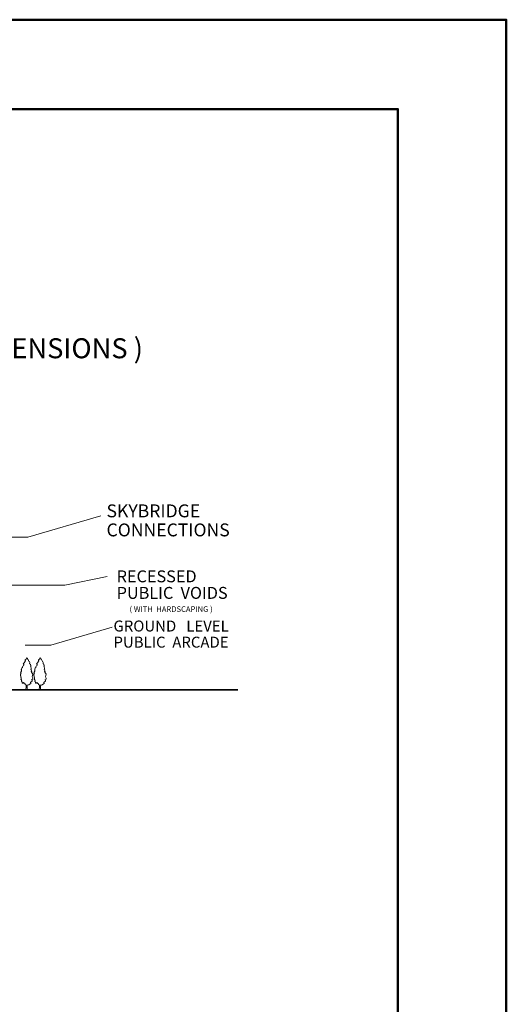
# Model space of a CAD drawing. Units: inches. Extents: x -1080 to 1950, y -1929 to 857.
# Tile 16 of 16: x 1335 to 1950, y -389 to 857. Entities that reach past the tile are written whole.
import ezdxf

# ---------------------------------------------------------------- set-up
doc = ezdxf.new("R2010")
doc.units = ezdxf.units.IN
doc.header["$MEASUREMENT"] = 0
for name, color, linetype, lineweight in [('A-ANNO-SYMB', 2, 'Continuous', 18), ('A-ANNO-TEXT', 7, 'Continuous', 25), ('A-ANNO-TTLB', 7, 'Continuous', 50), ('A-ELEV', 7, 'Continuous', 35), ('L-PLNT', 82, 'Continuous', 13)]:
    doc.layers.add(name, color=color, linetype=linetype, lineweight=lineweight)
doc.styles.get("Standard").update_dxf_attribs({"font": 'arial.ttf'})

# ---------------------------------------------------------------- blocks, each defined once
blk = doc.blocks.new('*U8')
blk.add_lwpolyline([(-69.9516, 4869.1546), (-172.212, 4644.4154), (-347.5228, 4494.6062), (-303.6824, 4400.9564), (-245.2624, 4382.2366), (-362.1278, 4326.0518), (-347.5228, 4251.1472), (-552.0182, 4007.6882), (-639.6736, 3932.7836), (-537.4132, 3820.414), (-552.0182, 3745.5094), (-581.2536, 3576.955), (-668.8836, 3558.2098), (-741.934, 3427.1204), (-727.329, 3277.3112), (-829.5894, 3258.5914), (-917.2194, 3052.572), (-873.4044, 3015.1324), (-902.6144, 2827.8582), (-990.2698, 2696.7434), (-873.4044, 2734.2084), (-1034.0848, 2509.4692), (-946.4294, 2434.5646), (-1034.0848, 2303.4752), (-1048.6898, 2041.2964), (-975.6648, 1985.1116), (-931.8244, 1797.8374), (-1004.8748, 1816.5572), (-946.4294, 1629.283), (-975.6648, 1460.7286), (-917.2194, 1479.4738), (-844.1944, 1329.6392), (-902.6144, 1348.3844), (-888.0094, 1179.83), (-771.144, 1142.365), (-800.354, 917.6512), (-668.8836, 936.371), (-595.8586, 1011.2756), (-464.3882, 917.6512), (-508.2032, 842.7212), (-376.7328, 805.2816), (-303.6824, 842.7212), (-318.2874, 692.912), (-157.607, 580.5424), (-99.187, 618.0074), (3.0734, 580.5424), (207.5942, 674.1922), (295.2496, 636.7272), (309.8546, 692.912), (543.56, 880.1862), (499.745, 992.5558), (602.0054, 1142.365), (762.6858, 1217.2696), (777.2908, 1367.1042), (645.8204, 1442.0088), (835.7362, 1554.3784), (864.9462, 1704.1876), (777.2908, 1910.207), (879.5512, 2284.7554), (675.0304, 2621.8388), (602.0054, 2621.8388), (718.8708, 2734.2084), (602.0054, 2809.113), (675.0304, 2940.2024), (645.8204, 2996.3872), (528.955, 3015.1324), (616.6104, 3164.9416), (572.7954, 3502.0504), (485.14, 3539.49), (572.7954, 3576.955), (499.745, 3857.8536), (368.2746, 3895.3186), (412.0896, 4120.0578), (309.8546, 4326.0518), (266.0142, 4251.1472), (149.1488, 4550.791), (105.3338, 4513.326), (17.6784, 4756.785), (-11.5316, 4719.32)], close=True)
for points in [[(-173.0502, 601.1926), (-173.0502, 296.3926), (-219.1258, 0)], [(9.8298, 601.1926), (-14.6304, 337.0834), (-14.6304, 93.6244), (0, 0)]]:
    blk.add_lwpolyline(points)
blk = doc.blocks.new('*U9')
blk.add_lwpolyline([(-69.9516, 4869.1546), (-172.212, 4644.4154), (-347.5228, 4494.6062), (-303.6824, 4400.9564), (-245.2624, 4382.2366), (-362.1278, 4326.0518), (-347.5228, 4251.1472), (-552.0182, 4007.6882), (-639.6736, 3932.7836), (-537.4132, 3820.414), (-552.0182, 3745.5094), (-581.2536, 3576.955), (-668.8836, 3558.2098), (-741.934, 3427.1204), (-727.329, 3277.3112), (-829.5894, 3258.5914), (-917.2194, 3052.572), (-873.4044, 3015.1324), (-902.6144, 2827.8582), (-990.2698, 2696.7434), (-873.4044, 2734.2084), (-1034.0848, 2509.4692), (-946.4294, 2434.5646), (-1034.0848, 2303.4752), (-1048.6898, 2041.2964), (-975.6648, 1985.1116), (-931.8244, 1797.8374), (-1004.8748, 1816.5572), (-946.4294, 1629.283), (-975.6648, 1460.7286), (-917.2194, 1479.4738), (-844.1944, 1329.6392), (-902.6144, 1348.3844), (-888.0094, 1179.83), (-771.144, 1142.365), (-800.354, 917.6512), (-668.8836, 936.371), (-595.8586, 1011.2756), (-464.3882, 917.6512), (-508.2032, 842.7212), (-376.7328, 805.2816), (-303.6824, 842.7212), (-318.2874, 692.912), (-157.607, 580.5424), (-99.187, 618.0074), (3.0734, 580.5424), (207.5942, 674.1922), (295.2496, 636.7272), (309.8546, 692.912), (543.56, 880.1862), (499.745, 992.5558), (602.0054, 1142.365), (762.6858, 1217.2696), (777.2908, 1367.1042), (645.8204, 1442.0088), (835.7362, 1554.3784), (864.9462, 1704.1876), (777.2908, 1910.207), (879.5512, 2284.7554), (675.0304, 2621.8388), (602.0054, 2621.8388), (718.8708, 2734.2084), (602.0054, 2809.113), (675.0304, 2940.2024), (645.8204, 2996.3872), (528.955, 3015.1324), (616.6104, 3164.9416), (572.7954, 3502.0504), (485.14, 3539.49), (572.7954, 3576.955), (499.745, 3857.8536), (368.2746, 3895.3186), (412.0896, 4120.0578), (309.8546, 4326.0518), (266.0142, 4251.1472), (149.1488, 4550.791), (105.3338, 4513.326), (17.6784, 4756.785), (-11.5316, 4719.32)], close=True)
for points in [[(-173.0502, 601.1926), (-173.0502, 296.3926), (-219.1258, 0)], [(9.8298, 601.1926), (-14.6304, 337.0834), (-14.6304, 93.6244), (0, 0)]]:
    blk.add_lwpolyline(points)

msp = doc.modelspace()

# ---------------------------------------------------------------- linework, layer by layer
at = {"layer": 'A-ANNO-SYMB'}
for p, q in [((1345.5, 202.1), (1438.1, 229)), ((1299.6, 202.1), (1345.5, 202.1)), ((1392.2, 141.5), (1445.8, 152.3)), ((1303.8, 141.5), (1392.2, 141.5)), ((1374.9, 65.8), (1452.2, 88.4)), ((1342.1, 65.8), (1374.9, 65.8))]:
    msp.add_line(p, q, dxfattribs=at)
at = {"layer": 'A-ANNO-TTLB'}
for points in [[(-1080.1, 856.5), (1950.4, 856.5), (1950.4, -1929), (-1080.1, -1929)], [(-957.6, 743.5), (1813.4, 743.5), (1813.4, -1770.5), (-957.6, -1770.5)]]:
    msp.add_lwpolyline(points, close=True, dxfattribs=at)
at = {"layer": 'A-ELEV'}
for p, q in [((887.3, 9), (1380.8, 9)), ((1380.8, 9), (1611.1, 9))]:
    msp.add_line(p, q, dxfattribs=at)

# ---------------------------------------------------------------- block references
at = {"layer": 'L-PLNT', "xscale": 0.0081804086702915, "yscale": 0.0081804086702915, "zscale": 0.0081804086702915}
for name, p in [('*U8', (1344.9, 10.1)), ('*U9', (1361.8, 10.1))]:
    msp.add_blockref(name, p, dxfattribs=at)

# ---------------------------------------------------------------- texts
at = {"layer": 'A-ANNO-TEXT'}
for s, height, p in [('PROPOSED   COMPLEX   INSTITUTIONAL   FACILITY - MODULAR   RESEARCH   AND   INNOVATION   AXIS   ( CONCEPTUAL   ONLY - NO   DIMENSIONS )', 25.272, (-818.2, 428.4)), ('SKYBRIDGE', 16.29, (1445.1, 227.3)), ('CONNECTIONS', 16.293, (1445.1, 203.2)), ('RECESSED', 15.06, (1457.9, 145.1)), ('PUBLIC  VOIDS', 15.063, (1457.9, 124.2)), ('( WITH  HARDSCAPING )', 7.055, (1474.2, 107.7)), ('GROUND   LEVEL ', 13.851, (1453.9, 82.9)), ('PUBLIC  ARCADE', 13.851, (1453.9, 62.5))]:
    msp.add_text(s, height=height, dxfattribs=at).set_placement(p)

doc.saveas('drawing.dxf')
